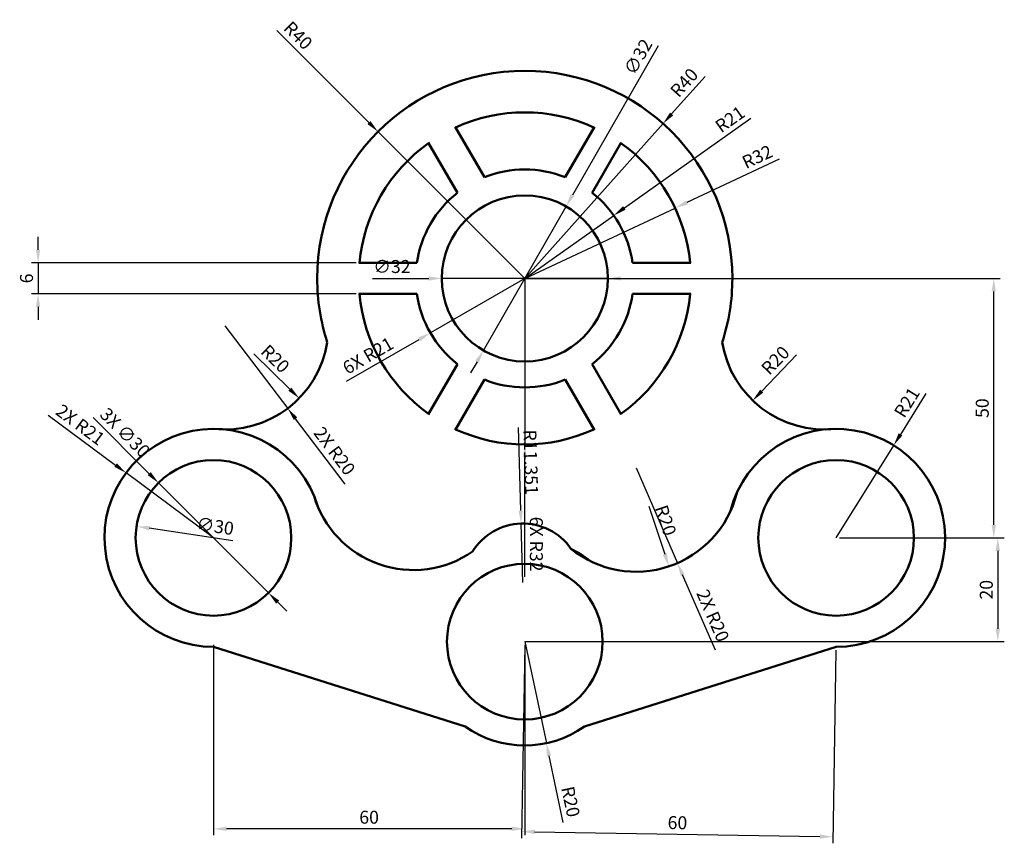
# Model space of a CAD drawing. Units: millimetres. Extents: x 2651 to 2841, y 1516 to 1675.
import ezdxf

# ---------------------------------------------------------------- set-up
doc = ezdxf.new("R2010")
doc.units = ezdxf.units.MM
doc.layers.add('M-DIMS', color=2, linetype='Continuous', lineweight=25)
doc.layers.add('M-OUTL', color=7, linetype='Continuous', lineweight=50)
doc.styles.get("Standard").update_dxf_attribs({"font": 'arial.ttf'})
doc.dimstyles.new('ISO-25', dxfattribs={"dimtxt": 2.5, "dimasz": 2.5, "dimexe": 1.25, "dimexo": 0.625, "dimtad": 1, "dimtxsty": 'Standard', "dimcen": 2.5, "dimadec": 0, "dimazin": 0, "dimtfac": 1, "dimtmove": 0, "dimatfit": 3, "dimfxl": 1, "dimarcsym": 0})

# ---------------------------------------------------------------- blocks, each defined once
blk = doc.blocks.new('*U1')
for p, q in [((-5.61, 3), (5.61, 3)), ((-5.61, -3), (5.61, -3))]:
    blk.add_line(p, q)
blk = doc.blocks.new('*U2')
at = {"layer": 'M-OUTL', "color": 0, "linetype": 'ByBlock', "lineweight": -2, "transparency": 16777216}
for p, rotation in [((2735.25, 1647.51), 119.9999999999999), ((2761.64, 1647.51), 59.99999999999997), ((2722.05, 1624.66), 180), ((2735.25, 1601.8), 239.9999999999999), ((2761.64, 1601.8), 299.9999999999999)]:
    blk.add_blockref('*U1', p, dxfattribs=dict(at, rotation=rotation))
blk.add_blockref('*U1', (2774.84, 1624.66), dxfattribs=at)
blk = doc.blocks.new('*D3')
at = {"layer": 'Defpoints', "color": 0, "transparency": 16777216}
for p in [(2756.4, 1638.54), (2740.48, 1610.78)]:
    blk.add_point(p, dxfattribs=at)
at = {"layer": 'M-DIMS', "color": 0, "lineweight": -2, "transparency": 16777216}
for p, q in [((2774.15, 1669.49), (2757.65, 1640.71)), ((2740.48, 1610.78), (2756.4, 1638.54)), ((2739.24, 1608.61), (2738, 1606.44))]:
    blk.add_line(p, q, dxfattribs=at)
blk.add_arc((2748.44, 1624.66), 16, 55.6937, 65.9751, dxfattribs=at)
at = {"layer": 'M-DIMS', "color": 0, "transparency": 16777216}
for points in [[(2757.28, 1640.91), (2758.01, 1640.5), (2756.4, 1638.54)], [(2738.88, 1608.82), (2739.6, 1608.4), (2740.48, 1610.78)]]:
    blk.add_solid(points, dxfattribs=at)
at = {"layer": 'M-DIMS', "color": 0, "transparency": 16777216, "insert": (2770.57, 1667.21), "char_height": 2.5, "attachment_point": 5, "rotation": 60.1699}
blk.add_mtext('∅32', dxfattribs=at)
blk = doc.blocks.new('*D4')
at = {"layer": 'Defpoints', "color": 0, "transparency": 16777216}
for p in [(2765.59, 1636.79), (2748.44, 1624.66)]:
    blk.add_point(p, dxfattribs=at)
at = {"layer": 'M-DIMS', "color": 0, "lineweight": -2, "transparency": 16777216}
for p, q in [((2792.02, 1655.49), (2767.63, 1638.23)), ((2748.44, 1624.66), (2765.59, 1636.79))]:
    blk.add_line(p, q, dxfattribs=at)
at = {"layer": 'M-DIMS', "color": 0, "transparency": 16777216}
blk.add_solid([(2767.39, 1638.57), (2767.87, 1637.89), (2765.59, 1636.79)], dxfattribs=at)
at = {"layer": 'M-DIMS', "color": 0, "transparency": 16777216, "insert": (2788.18, 1655.07), "char_height": 2.5, "attachment_point": 5, "rotation": 35.2761}
blk.add_mtext('R21', dxfattribs=at)
blk = doc.blocks.new('*D5')
at = {"layer": 'Defpoints', "color": 0, "transparency": 16777216}
for p in [(2777.42, 1638.23), (2748.44, 1624.66)]:
    blk.add_point(p, dxfattribs=at)
at = {"layer": 'M-DIMS', "color": 0, "lineweight": -2, "transparency": 16777216}
for p, q in [((2797.45, 1647.61), (2779.69, 1639.29)), ((2748.44, 1624.66), (2777.42, 1638.23))]:
    blk.add_line(p, q, dxfattribs=at)
at = {"layer": 'M-DIMS', "color": 0, "transparency": 16777216}
blk.add_solid([(2779.51, 1639.67), (2779.86, 1638.91), (2777.42, 1638.23)], dxfattribs=at)
at = {"layer": 'M-DIMS', "color": 0, "transparency": 16777216, "insert": (2793.38, 1647.81), "char_height": 2.5, "attachment_point": 5, "rotation": 25.0956}
blk.add_mtext('R32', dxfattribs=at)
blk = doc.blocks.new('*D6')
at = {"layer": 'Defpoints', "color": 0, "transparency": 16777216}
for p in [(2775.09, 1654.49), (2748.44, 1624.66)]:
    blk.add_point(p, dxfattribs=at)
at = {"layer": 'M-DIMS', "color": 0, "lineweight": -2, "transparency": 16777216}
for p, q in [((2783.23, 1663.6), (2776.75, 1656.35)), ((2748.44, 1624.66), (2775.09, 1654.49))]:
    blk.add_line(p, q, dxfattribs=at)
at = {"layer": 'M-DIMS', "color": 0, "transparency": 16777216}
blk.add_solid([(2776.44, 1656.63), (2777.06, 1656.08), (2775.09, 1654.49)], dxfattribs=at)
at = {"layer": 'M-DIMS', "color": 0, "transparency": 16777216, "insert": (2779.4, 1662.18), "char_height": 2.5, "attachment_point": 5, "rotation": 48.2294}
blk.add_mtext('R40', dxfattribs=at)
blk = doc.blocks.new('*D7')
at = {"layer": 'Defpoints', "color": 0, "transparency": 16777216}
for p in [(2769.89, 1588.14), (2776.22, 1569.17)]:
    blk.add_point(p, dxfattribs=at)
at = {"layer": 'M-DIMS', "color": 0, "lineweight": -2, "transparency": 16777216}
blk.add_line((2772.36, 1580.75), (2775.43, 1571.54), dxfattribs=at)
at = {"layer": 'M-DIMS', "color": 0, "transparency": 16777216}
blk.add_solid([(2775.82, 1571.67), (2775.03, 1571.41), (2776.22, 1569.17)], dxfattribs=at)
at = {"layer": 'M-DIMS', "color": 0, "transparency": 16777216, "insert": (2775.3, 1577.93), "char_height": 2.5, "attachment_point": 5, "rotation": 288.4301}
blk.add_mtext('R20', dxfattribs=at)
blk = doc.blocks.new('*D8')
at = {"layer": 'Defpoints', "color": 0, "transparency": 16777216}
for p in [(2673.61, 1576.89), (2703.28, 1572.42)]:
    blk.add_point(p, dxfattribs=at)
at = {"layer": 'M-DIMS', "color": 0, "lineweight": -2, "transparency": 16777216}
blk.add_line((2692.17, 1574.1), (2676.08, 1576.52), dxfattribs=at)
blk.add_arc((2688.44, 1574.66), 15, 166.6539, 194.2058, dxfattribs=at)
at = {"layer": 'M-DIMS', "color": 0, "transparency": 16777216}
blk.add_solid([(2676.14, 1576.93), (2676.02, 1576.11), (2673.61, 1576.89)], dxfattribs=at)
at = {"layer": 'M-DIMS', "color": 0, "transparency": 16777216, "insert": (2688.74, 1576.61), "char_height": 2.5, "attachment_point": 5, "rotation": 351.4286}
blk.add_mtext('∅30', dxfattribs=at)
blk = doc.blocks.new('*D9')
at = {"layer": 'Defpoints', "color": 0, "transparency": 16777216}
for p in [(2690.64, 1615.54), (2704.96, 1601.57)]:
    blk.add_point(p, dxfattribs=at)
at = {"layer": 'M-DIMS', "color": 0, "lineweight": -2, "transparency": 16777216}
blk.add_line((2696.21, 1610.1), (2703.17, 1603.31), dxfattribs=at)
at = {"layer": 'M-DIMS', "color": 0, "transparency": 16777216}
blk.add_solid([(2703.46, 1603.61), (2702.88, 1603.01), (2704.96, 1601.57)], dxfattribs=at)
at = {"layer": 'M-DIMS', "color": 0, "transparency": 16777216, "insert": (2700.12, 1608.94), "char_height": 2.5, "attachment_point": 5, "rotation": 315.6948}
blk.add_mtext('R20', dxfattribs=at)
blk = doc.blocks.new('*D10')
at = {"layer": 'Defpoints', "color": 0, "transparency": 16777216}
for p in [(2806.24, 1615.54), (2792.37, 1601.13)]:
    blk.add_point(p, dxfattribs=at)
at = {"layer": 'M-DIMS', "color": 0, "lineweight": -2, "transparency": 16777216}
blk.add_line((2800.84, 1609.93), (2794.1, 1602.93), dxfattribs=at)
at = {"layer": 'M-DIMS', "color": 0, "transparency": 16777216}
blk.add_solid([(2793.8, 1603.22), (2794.4, 1602.64), (2792.37, 1601.13)], dxfattribs=at)
at = {"layer": 'M-DIMS', "color": 0, "transparency": 16777216, "insert": (2796.97, 1608.65), "char_height": 2.5, "attachment_point": 5, "rotation": 46.0717}
blk.add_mtext('R20', dxfattribs=at)
blk = doc.blocks.new('*D11')
at = {"layer": 'Defpoints', "color": 0, "transparency": 16777216}
for p in [(2819.54, 1592.49), (2808.44, 1574.66)]:
    blk.add_point(p, dxfattribs=at)
at = {"layer": 'M-DIMS', "color": 0, "lineweight": -2, "transparency": 16777216}
for p, q in [((2825.74, 1602.46), (2820.86, 1594.61)), ((2808.44, 1574.66), (2819.54, 1592.49))]:
    blk.add_line(p, q, dxfattribs=at)
at = {"layer": 'M-DIMS', "color": 0, "transparency": 16777216}
blk.add_solid([(2820.5, 1594.83), (2821.21, 1594.39), (2819.54, 1592.49)], dxfattribs=at)
at = {"layer": 'M-DIMS', "color": 0, "transparency": 16777216, "insert": (2822.36, 1600.59), "char_height": 2.5, "attachment_point": 5, "rotation": 58.1148}
blk.add_mtext('R21', dxfattribs=at)
blk = doc.blocks.new('*D12')
at = {"layer": 'Defpoints', "color": 0, "transparency": 16777216}
for p in [(2808.44, 1624.66), (2838.83, 1624.66), (2808.44, 1574.66)]:
    blk.add_point(p, dxfattribs=at)
at = {"layer": 'M-DIMS', "color": 0, "lineweight": -2, "transparency": 16777216}
for p, q in [((2809.07, 1624.66), (2840.08, 1624.66)), ((2838.83, 1577.16), (2838.83, 1622.16)), ((2809.07, 1574.66), (2840.08, 1574.66))]:
    blk.add_line(p, q, dxfattribs=at)
at = {"layer": 'M-DIMS', "color": 0, "transparency": 16777216}
for points in [[(2838.42, 1622.16), (2839.25, 1622.16), (2838.83, 1624.66)], [(2838.42, 1577.16), (2839.25, 1577.16), (2838.83, 1574.66)]]:
    blk.add_solid(points, dxfattribs=at)
at = {"layer": 'M-DIMS', "color": 0, "transparency": 16777216, "insert": (2836.93, 1599.66), "char_height": 2.5, "attachment_point": 5, "rotation": 90}
blk.add_mtext('50', dxfattribs=at)
blk = doc.blocks.new('*D13')
at = {"layer": 'Defpoints', "color": 0, "transparency": 16777216}
for p in [(2838.83, 1574.66), (2838.83, 1554.66), (2839.61, 1554.66)]:
    blk.add_point(p, dxfattribs=at)
at = {"layer": 'M-DIMS', "color": 0, "lineweight": -2, "transparency": 16777216}
for p, q in [((2839.46, 1574.66), (2840.86, 1574.66)), ((2839.61, 1572.16), (2839.61, 1557.16)), ((2839.46, 1554.66), (2840.86, 1554.66))]:
    blk.add_line(p, q, dxfattribs=at)
at = {"layer": 'M-DIMS', "color": 0, "transparency": 16777216}
for points in [[(2839.19, 1572.16), (2840.02, 1572.16), (2839.61, 1574.66)], [(2839.19, 1557.16), (2840.02, 1557.16), (2839.61, 1554.66)]]:
    blk.add_solid(points, dxfattribs=at)
at = {"layer": 'M-DIMS', "color": 0, "transparency": 16777216, "insert": (2837.71, 1564.66), "char_height": 2.5, "attachment_point": 5, "rotation": 90}
blk.add_mtext('20', dxfattribs=at)
blk = doc.blocks.new('*D14')
at = {"layer": 'Defpoints', "color": 0, "transparency": 16777216}
for p in [(2748.44, 1554.66), (2808.43, 1553.66), (2807.82, 1517.05)]:
    blk.add_point(p, dxfattribs=at)
at = {"layer": 'M-DIMS', "color": 0, "lineweight": -2, "transparency": 16777216}
for p, q in [((2748.43, 1554.03), (2747.81, 1516.8)), ((2808.42, 1553.03), (2807.8, 1515.8)), ((2750.33, 1518), (2805.32, 1517.09))]:
    blk.add_line(p, q, dxfattribs=at)
at = {"layer": 'M-DIMS', "color": 0, "transparency": 16777216}
for points in [[(2750.34, 1518.42), (2750.33, 1517.59), (2747.83, 1518.05)], [(2805.33, 1517.5), (2805.32, 1516.67), (2807.82, 1517.05)]]:
    blk.add_solid(points, dxfattribs=at)
at = {"layer": 'M-DIMS', "color": 0, "transparency": 16777216, "insert": (2777.86, 1519.45), "char_height": 2.5, "attachment_point": 5, "rotation": 359.0452}
blk.add_mtext('60', dxfattribs=at)
blk = doc.blocks.new('*D15')
at = {"layer": 'Defpoints', "color": 0, "transparency": 16777216}
for p in [(2688.44, 1554.66), (2748.44, 1554.66), (2688.44, 1518.59)]:
    blk.add_point(p, dxfattribs=at)
at = {"layer": 'M-DIMS', "color": 0, "lineweight": -2, "transparency": 16777216}
for p, q in [((2688.44, 1554.03), (2688.44, 1517.34)), ((2748.44, 1554.03), (2748.44, 1517.34)), ((2745.94, 1518.59), (2690.94, 1518.59))]:
    blk.add_line(p, q, dxfattribs=at)
at = {"layer": 'M-DIMS', "color": 0, "transparency": 16777216}
for points in [[(2690.94, 1519.01), (2690.94, 1518.18), (2688.44, 1518.59)], [(2745.94, 1519.01), (2745.94, 1518.18), (2748.44, 1518.59)]]:
    blk.add_solid(points, dxfattribs=at)
at = {"layer": 'M-DIMS', "color": 0, "transparency": 16777216, "insert": (2718.44, 1520.5), "char_height": 2.5, "attachment_point": 5}
blk.add_mtext('60', dxfattribs=at)
blk = doc.blocks.new('MOUNT-HOLE-D30')
blk.add_circle((0, 0), 15)
blk = doc.blocks.new('ANNULAR-SLOT-ARCS-R21-R32')
for radius, start, end in [(32, 5.3794, 54.6206), (21, 8.2132, 51.7868)]:
    blk.add_arc((0, 0), radius, start, end)
blk = doc.blocks.new('*D18')
at = {"layer": 'Defpoints', "color": 0, "transparency": 16777216}
for p in [(2716.58, 1627.66), (2654.64, 1621.66), (2716.58, 1621.66)]:
    blk.add_point(p, dxfattribs=at)
at = {"layer": 'M-DIMS', "color": 0, "lineweight": -2, "transparency": 16777216}
for p, q in [((2654.64, 1630.16), (2654.64, 1632.66)), ((2715.96, 1627.66), (2653.39, 1627.66)), ((2654.64, 1627.66), (2654.64, 1621.66)), ((2715.96, 1621.66), (2653.39, 1621.66)), ((2654.64, 1619.16), (2654.64, 1616.66))]:
    blk.add_line(p, q, dxfattribs=at)
at = {"layer": 'M-DIMS', "color": 0, "transparency": 16777216}
for points in [[(2654.23, 1630.16), (2655.06, 1630.16), (2654.64, 1627.66)], [(2654.23, 1619.16), (2655.06, 1619.16), (2654.64, 1621.66)]]:
    blk.add_solid(points, dxfattribs=at)
at = {"layer": 'M-DIMS', "color": 0, "transparency": 16777216, "insert": (2652.74, 1624.66), "char_height": 2.5, "attachment_point": 5, "rotation": 90}
blk.add_mtext('6', dxfattribs=at)
blk = doc.blocks.new('*D19')
at = {"layer": 'Defpoints', "color": 0, "transparency": 16777216}
for p in [(2677.84, 1585.26), (2699.05, 1564.05)]:
    blk.add_point(p, dxfattribs=at)
at = {"layer": 'M-DIMS', "color": 0, "lineweight": -2, "transparency": 16777216}
for p, q in [((2665.26, 1597.84), (2676.07, 1587.03)), ((2699.05, 1564.05), (2677.84, 1585.26)), ((2700.82, 1562.28), (2702.58, 1560.51))]:
    blk.add_line(p, q, dxfattribs=at)
at = {"layer": 'M-DIMS', "color": 0, "transparency": 16777216}
for points in [[(2676.36, 1587.33), (2675.77, 1586.74), (2677.84, 1585.26)], [(2701.11, 1562.58), (2700.52, 1561.99), (2699.05, 1564.05)]]:
    blk.add_solid(points, dxfattribs=at)
at = {"layer": 'M-DIMS', "color": 0, "transparency": 16777216, "insert": (2671.18, 1594.71), "char_height": 2.5, "attachment_point": 5, "rotation": 314.9981}
blk.add_mtext('3X ∅30', dxfattribs=at)
blk = doc.blocks.new('*D20')
at = {"layer": 'Defpoints', "color": 0, "transparency": 16777216}
for p in [(2732.44, 1624.66), (2764.44, 1624.66)]:
    blk.add_point(p, dxfattribs=at)
at = {"layer": 'M-DIMS', "color": 0, "lineweight": -2, "transparency": 16777216}
for p, q in [((2719.08, 1624.66), (2729.94, 1624.66)), ((2764.44, 1624.66), (2732.44, 1624.66)), ((2766.94, 1624.66), (2769.44, 1624.66))]:
    blk.add_line(p, q, dxfattribs=at)
at = {"layer": 'M-DIMS', "color": 0, "transparency": 16777216}
for points in [[(2729.94, 1625.07), (2729.94, 1624.24), (2732.44, 1624.66)], [(2766.94, 1625.07), (2766.94, 1624.24), (2764.44, 1624.66)]]:
    blk.add_solid(points, dxfattribs=at)
at = {"layer": 'M-DIMS', "color": 0, "transparency": 16777216, "insert": (2722.84, 1626.63), "char_height": 2.5, "attachment_point": 5, "rotation": 359.9984}
blk.add_mtext('∅32', dxfattribs=at)
blk = doc.blocks.new('*D21')
at = {"layer": 'Defpoints', "color": 0, "transparency": 16777216}
for p in [(2720.16, 1652.94), (2748.44, 1624.66)]:
    blk.add_point(p, dxfattribs=at)
at = {"layer": 'M-DIMS', "color": 0, "lineweight": -2, "transparency": 16777216}
for p, q in [((2700.64, 1672.46), (2718.39, 1654.71)), ((2748.44, 1624.66), (2720.16, 1652.94))]:
    blk.add_line(p, q, dxfattribs=at)
at = {"layer": 'M-DIMS', "color": 0, "transparency": 16777216}
blk.add_solid([(2718.69, 1655), (2718.1, 1654.41), (2720.16, 1652.94)], dxfattribs=at)
at = {"layer": 'M-DIMS', "color": 0, "transparency": 16777216, "insert": (2704.53, 1671.26), "char_height": 2.5, "attachment_point": 5, "rotation": 315.0003}
blk.add_mtext('R40', dxfattribs=at)
blk = doc.blocks.new('*D22')
at = {"layer": 'Defpoints', "color": 0, "transparency": 16777216}
for p in [(2748.44, 1624.66), (2748.44, 1592.66)]:
    blk.add_point(p, dxfattribs=at)
at = {"layer": 'M-DIMS', "color": 0, "lineweight": -2, "transparency": 16777216}
for p, q in [((2748.44, 1624.66), (2748.44, 1592.66)), ((2748.44, 1567.17), (2748.44, 1590.16))]:
    blk.add_line(p, q, dxfattribs=at)
at = {"layer": 'M-DIMS', "color": 0, "transparency": 16777216}
blk.add_solid([(2748.86, 1590.16), (2748.03, 1590.16), (2748.44, 1592.66)], dxfattribs=at)
at = {"layer": 'M-DIMS', "color": 0, "transparency": 16777216, "insert": (2750.35, 1573.46), "char_height": 2.5, "attachment_point": 5, "rotation": 270.0004}
blk.add_mtext('6X R32', dxfattribs=at)
blk = doc.blocks.new('*D23')
at = {"layer": 'Defpoints', "color": 0, "transparency": 16777216}
for p in [(2748.44, 1624.66), (2730.26, 1614.16)]:
    blk.add_point(p, dxfattribs=at)
at = {"layer": 'M-DIMS', "color": 0, "lineweight": -2, "transparency": 16777216}
for p, q in [((2748.44, 1624.66), (2730.26, 1614.16)), ((2714.09, 1604.83), (2728.09, 1612.91))]:
    blk.add_line(p, q, dxfattribs=at)
at = {"layer": 'M-DIMS', "color": 0, "transparency": 16777216}
blk.add_solid([(2727.88, 1613.27), (2728.3, 1612.55), (2730.26, 1614.16)], dxfattribs=at)
at = {"layer": 'M-DIMS', "color": 0, "transparency": 16777216, "insert": (2718.39, 1609.5), "char_height": 2.5, "attachment_point": 5, "rotation": 29.9986}
blk.add_mtext('6X R21', dxfattribs=at)
blk = doc.blocks.new('*D24')
at = {"layer": 'Defpoints', "color": 0, "transparency": 16777216}
for p in [(2671.59, 1587.19), (2688.44, 1574.66)]:
    blk.add_point(p, dxfattribs=at)
at = {"layer": 'M-DIMS', "color": 0, "lineweight": -2, "transparency": 16777216}
for p, q in [((2656.6, 1598.33), (2669.58, 1588.68)), ((2688.44, 1574.66), (2671.59, 1587.19))]:
    blk.add_line(p, q, dxfattribs=at)
at = {"layer": 'M-DIMS', "color": 0, "transparency": 16777216}
blk.add_solid([(2669.83, 1589.01), (2669.34, 1588.34), (2671.59, 1587.19)], dxfattribs=at)
at = {"layer": 'M-DIMS', "color": 0, "transparency": 16777216, "insert": (2662.6, 1596.21), "char_height": 2.5, "attachment_point": 5, "rotation": 323.3705}
blk.add_mtext('2X R21', dxfattribs=at)
blk = doc.blocks.new('*D25')
at = {"layer": 'Defpoints', "color": 0, "transparency": 16777216}
for p in [(2690.64, 1615.54), (2702.75, 1599.61)]:
    blk.add_point(p, dxfattribs=at)
at = {"layer": 'M-DIMS', "color": 0, "lineweight": -2, "transparency": 16777216}
for p, q in [((2690.64, 1615.54), (2702.75, 1599.61)), ((2713.83, 1585.03), (2704.26, 1597.62))]:
    blk.add_line(p, q, dxfattribs=at)
at = {"layer": 'M-DIMS', "color": 0, "transparency": 16777216}
blk.add_solid([(2704.59, 1597.88), (2703.93, 1597.37), (2702.75, 1599.61)], dxfattribs=at)
at = {"layer": 'M-DIMS', "color": 0, "transparency": 16777216, "insert": (2711.52, 1591.21), "char_height": 2.5, "attachment_point": 5, "rotation": 307.2424}
blk.add_mtext('2X R20', dxfattribs=at)
blk = doc.blocks.new('*D26')
at = {"layer": 'Defpoints', "color": 0, "transparency": 16777216}
for p in [(2769.89, 1588.14), (2777.87, 1569.8)]:
    blk.add_point(p, dxfattribs=at)
at = {"layer": 'M-DIMS', "color": 0, "lineweight": -2, "transparency": 16777216}
for p, q in [((2769.89, 1588.14), (2777.87, 1569.8)), ((2785.17, 1553), (2778.87, 1567.51))]:
    blk.add_line(p, q, dxfattribs=at)
at = {"layer": 'M-DIMS', "color": 0, "transparency": 16777216}
blk.add_solid([(2779.25, 1567.67), (2778.48, 1567.34), (2777.87, 1569.8)], dxfattribs=at)
at = {"layer": 'M-DIMS', "color": 0, "transparency": 16777216, "insert": (2784.4, 1559.55), "char_height": 2.5, "attachment_point": 5, "rotation": 293.5026}
blk.add_mtext('2X R20', dxfattribs=at)
blk = doc.blocks.new('*D27')
at = {"layer": 'Defpoints', "color": 0, "transparency": 16777216}
for p in [(2747.72, 1577.41), (2748.04, 1566.06)]:
    blk.add_point(p, dxfattribs=at)
at = {"layer": 'M-DIMS', "color": 0, "lineweight": -2, "transparency": 16777216}
for p, q in [((2747.18, 1595.94), (2747.64, 1579.91)), ((2748.04, 1566.06), (2747.72, 1577.41))]:
    blk.add_line(p, q, dxfattribs=at)
at = {"layer": 'M-DIMS', "color": 0, "transparency": 16777216}
blk.add_solid([(2748.06, 1579.92), (2747.23, 1579.9), (2747.72, 1577.41)], dxfattribs=at)
at = {"layer": 'M-DIMS', "color": 0, "transparency": 16777216, "insert": (2749.28, 1589.23), "char_height": 2.5, "attachment_point": 5, "rotation": 271.6425}
blk.add_mtext('R11.351', dxfattribs=at)
blk = doc.blocks.new('*D28')
at = {"layer": 'Defpoints', "color": 0, "transparency": 16777216}
for p in [(2748.44, 1554.66), (2752.6, 1535.09)]:
    blk.add_point(p, dxfattribs=at)
at = {"layer": 'M-DIMS', "color": 0, "lineweight": -2, "transparency": 16777216}
for p, q in [((2748.44, 1554.66), (2752.6, 1535.09)), ((2755.85, 1519.83), (2753.12, 1532.65))]:
    blk.add_line(p, q, dxfattribs=at)
at = {"layer": 'M-DIMS', "color": 0, "transparency": 16777216}
blk.add_solid([(2753.53, 1532.74), (2752.71, 1532.56), (2752.6, 1535.09)], dxfattribs=at)
at = {"layer": 'M-DIMS', "color": 0, "transparency": 16777216, "insert": (2756.96, 1523.75), "char_height": 2.5, "attachment_point": 5, "rotation": 282.0004}
blk.add_mtext('R20', dxfattribs=at)

msp = doc.modelspace()

# ---------------------------------------------------------------- linework, layer by layer
at = {"layer": 'M-DIMS'}
for p, q in [((2748.4428, 1624.6576), (2819.5335, 1624.6576)), ((2748.4428, 1554.6576), (2839.6078, 1554.6576))]:
    msp.add_line(p, q, dxfattribs=at)
at = {"layer": 'M-OUTL'}
for p, q in [((2688.4428, 1553.6576), (2736.9305, 1538.3031)), ((2808.4428, 1553.6576), (2759.955, 1538.3031))]:
    msp.add_line(p, q, dxfattribs=at)
msp.add_circle((2748.4428, 1624.6576), 16, dxfattribs=at)
for centre, radius, start, end in [((2748.4428, 1624.6576), 40, 0, 180), ((2748.4428, 1624.6576), 40, 180, 197.936292), ((2748.4428, 1624.6576), 40, 342.063708, 0), ((2690.6439, 1615.5361), 20, 263.681306, 350.802175), ((2806.2416, 1615.5361), 20, 189.197825, 276.318694), ((2688.4428, 1574.6576), 21, 16.741391, 270), ((2808.4428, 1574.6576), 21, 270, 165.685916), ((2726.988, 1588.4614), 20, 196.593142, 304.722969), ((2769.894, 1588.1402), 20, 231.137925, 345.934761), ((2748.0414, 1566.0637), 11.3513, 34.953473, 148.332073), ((2748.4428, 1554.6576), 20, 51.137925, 63.569293), ((2748.4428, 1554.6576), 20, 234.857482, 305.142518)]:
    msp.add_arc(centre, radius, start, end, dxfattribs=at)

# ---------------------------------------------------------------- block references
for rotation in [59.99999999999758, 119.9999999999987, 299.9999999999994, 180, 239.9999999999991]:
    msp.add_blockref('ANNULAR-SLOT-ARCS-R21-R32', (2748.4428, 1624.6576), dxfattribs=dict(at, rotation=rotation))
for name, p in [('*U2', (0, 0)), ('ANNULAR-SLOT-ARCS-R21-R32', (2748.4428, 1624.6576)), ('MOUNT-HOLE-D30', (2688.4428, 1574.6576)), ('MOUNT-HOLE-D30', (2808.4428, 1574.6576)), ('MOUNT-HOLE-D30', (2748.4428, 1554.6576))]:
    msp.add_blockref(name, p, dxfattribs=at)

# ---------------------------------------------------------------- dimensions: what is measured, and where the dimension line sits
at = {"layer": 'M-DIMS'}
for center, mpoint, override, picture, middle in [((2748.4428, 1624.6576), (2720.1583, 1652.9417), {"dimdec": 0, "dimlfac": 1, "dimrnd": 0, "dimzin": 0, "dimdsep": 46, "dimlunit": 2}, '*D21', (2703.1877, 1669.9121)), ((2748.4428, 1624.6576), (2765.5867, 1636.7854), {"dimclrd": 0, "dimclre": 0, "dimclrt": 0}, '*D4', (2789.2692, 1653.5387)), ((2748.4428, 1624.6576), (2777.422, 1638.2297), {"dimclrd": 0, "dimclre": 0, "dimclrt": 0}, '*D5', (2794.1914, 1646.0835)), ((2690.6439, 1615.5361), (2704.9565, 1601.5665), {"dimclrd": 0, "dimclre": 0, "dimclrt": 0}, '*D9', (2698.7967, 1607.5787)), ((2806.2416, 1615.5361), (2792.3664, 1601.1319), {"dimclrd": 0, "dimclre": 0, "dimclrt": 0}, '*D10', (2798.338, 1607.3312)), ((2769.894, 1588.1402), (2776.217, 1569.166), {"dimclrd": 0, "dimclre": 0, "dimclrt": 0}, '*D7', (2773.4957, 1577.3321)), ((2748.4428, 1554.6576), (2752.6011, 1535.0946), {"dimdec": 0, "dimlfac": 1, "dimrnd": 0, "dimzin": 0, "dimdsep": 46, "dimlunit": 2}, '*D28', (2755.0962, 1523.3569))]:
    dim = msp.add_radius_dim(center=center, mpoint=mpoint, dimstyle='ISO-25', override=override, dxfattribs=at)
    dim.commit()
    dim.dimension.update_dxf_attribs({"geometry": picture, "text_midpoint": middle, "dimtype": 164})
for p1, p2, override, picture, middle in [((2740.4839, 1610.7775), (2756.4016, 1638.5376), {"dimclrd": 0, "dimclre": 0, "dimclrt": 0}, '*D3', (2772.2796, 1666.2284)), ((2764.4428, 1624.6571), (2732.4428, 1624.658), {"dimdec": 0, "dimlfac": 1, "dimrnd": 0, "dimzin": 0, "dimdsep": 46, "dimlunit": 2}, '*D20', (2722.8428, 1624.6583)), ((2703.2752, 1572.4219), (2673.6103, 1576.8932), {"dimclrd": 0, "dimclre": 0, "dimclrt": 0}, '*D8', (2688.4428, 1574.6576))]:
    dim = msp.add_diameter_dim_2p(p1=p1, p2=p2, dimstyle='ISO-25', override=override, dxfattribs=at)
    dim.commit()
    dim.dimension.update_dxf_attribs({"geometry": picture, "text_midpoint": middle, "dimtype": 163})
for center, mpoint, override, picture, middle in [((2748.4428, 1624.6576), (2775.0888, 1654.4903), {"dimclrd": 0, "dimclre": 0, "dimclrt": 0}, '*D6', (2779.4046, 1662.1766)), ((2808.4428, 1574.6576), (2819.5354, 1592.4888), {"dimclrd": 0, "dimclre": 0, "dimclrt": 0}, '*D11', (2822.3604, 1600.5895)), ((2748.0414, 1566.0637), (2747.716, 1577.4104), {"dimdec": 3, "dimlfac": 1, "dimrnd": 0, "dimzin": 0, "dimdsep": 46, "dimlunit": 2}, '*D27', (2749.2801, 1589.2293))]:
    dim = msp.add_radius_dim(center=center, mpoint=mpoint, dimstyle='ISO-25', override=override, dxfattribs=at)
    dim.commit()
    dim.dimension.update_dxf_attribs({"geometry": picture, "text_midpoint": middle})
for base, p1, p2, override, picture, middle in [((2654.6423, 1621.6576), (2716.5837, 1627.6576), (2716.5837, 1621.6576), {"dimdec": 0, "dimlfac": 1, "dimrnd": 0, "dimzin": 0, "dimdsep": 46, "dimlunit": 2}, '*D18', (2652.7409, 1624.6576)), ((2838.8347, 1624.6576), (2808.4428, 1574.6576), (2808.4428, 1624.6576), {"dimclrd": 0, "dimclre": 0, "dimclrt": 0}, '*D12', (2836.9333, 1599.6576)), ((2839.6078, 1554.6576), (2838.8347, 1574.6576), (2838.8347, 1554.6576), {"dimclrd": 0, "dimclre": 0, "dimclrt": 0}, '*D13', (2837.7063, 1564.6576))]:
    dim = msp.add_linear_dim(base=base, p1=p1, p2=p2, angle=90, dimstyle='ISO-25', override=override, dxfattribs=at)
    dim.commit()
    dim.dimension.update_dxf_attribs({"geometry": picture, "text_midpoint": middle})
for center, mpoint, text, picture, middle in [((2748.4428, 1624.6576), (2730.256, 1614.158), '6X <>', '*D23', (2719.3439, 1607.8582)), ((2748.4428, 1624.6576), (2748.443, 1592.6576), '6X <>', '*D22', (2748.4431, 1573.4576)), ((2690.6439, 1615.5361), (2702.7477, 1599.6144), '2X <>', '*D25', (2710.01, 1590.0614)), ((2688.4428, 1574.6576), (2671.59, 1587.187), '2X <>', '*D24', (2661.4784, 1594.7046)), ((2769.894, 1588.1402), (2777.8698, 1569.7994), '2X <>', '*D26', (2782.6553, 1558.7948))]:
    dim = msp.add_radius_dim(center=center, mpoint=mpoint, text=text, dimstyle='ISO-25', override={"dimdec": 0, "dimlfac": 1, "dimrnd": 0, "dimzin": 0, "dimdsep": 46, "dimlunit": 2}, dxfattribs=at)
    dim.commit()
    dim.dimension.update_dxf_attribs({"geometry": picture, "text_midpoint": middle, "dimtype": 164})
dim = msp.add_diameter_dim_2p(p1=(2699.049, 1564.0506), p2=(2677.8365, 1585.2645), text='3X <>', dimstyle='ISO-25', override={"dimdec": 0, "dimlfac": 1, "dimrnd": 0, "dimzin": 0, "dimdsep": 46, "dimlunit": 2}, dxfattribs=at)
dim.commit()
dim.dimension.update_dxf_attribs({"geometry": '*D19', "text_midpoint": (2669.7829, 1593.3186), "dimtype": 163})
dim = msp.add_linear_dim(base=(2688.4428, 1518.5938), p1=(2748.4428, 1554.6576), p2=(2688.4428, 1554.6576), dimstyle='ISO-25', override={"dimclrd": 0, "dimclre": 0, "dimclrt": 0}, dxfattribs=at)
dim.commit()
dim.dimension.update_dxf_attribs({"geometry": '*D15', "text_midpoint": (2718.4428, 1520.4952)})
dim = msp.add_aligned_dim(p1=(2748.4428, 1554.6576), p2=(2808.4344, 1553.6577), distance=-36.6175, dimstyle='ISO-25', override={"dimclrd": 0, "dimclre": 0, "dimclrt": 0}, dxfattribs=at)
dim.commit()
dim.dimension.update_dxf_attribs({"geometry": '*D14', "text_midpoint": (2777.8601, 1519.4464)})

doc.saveas('drawing.dxf')
